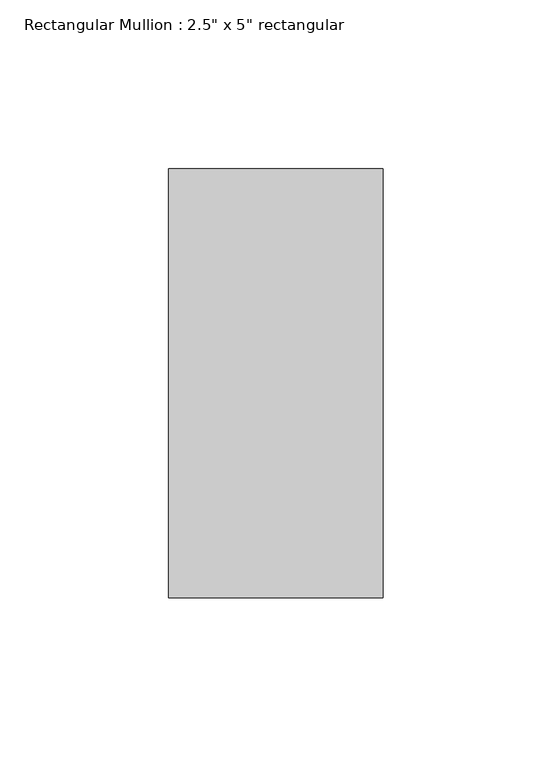
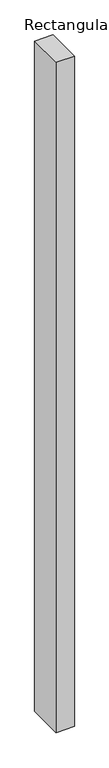
"""IFC4 building model written with IfcOpenShell, lengths in millimetres: member geometry."""

from ifc_helpers import new_model, si_unit, frame, origin, place, context, project, spatial, polyline, outline, extrude, source, transform, mapped, element, save


def member_8dcffc12(model_context):
    return source(origin(), model_context, "Body", "SweptSolid", [
        extrude(outline(polyline([(0.0, 63.5), (0.0, -63.5), (-63.5, -63.5), (-63.5, 63.5), (0.0, 63.5)])), frame((0.0, 0.0, -2445.9925421), z_axis=(0.0, 0.0, 1.0), x_axis=(1.0, 0.0, 0.0)), (0.0, 0.0, 1.0), 2445.9925421),
    ])


if __name__ == "__main__":
    model = new_model("IFC4")
    model_context = context("Model", 3, world=origin())
    ifc_project = project(units=[si_unit("LENGTHUNIT", "METRE", prefix="MILLI")], contexts=[model_context])
    site = spatial("IfcSite", under=ifc_project)
    building = spatial("IfcBuilding", under=site)
    placement = place(None, origin())
    member_shape = member_8dcffc12(model_context)
    element("IfcMember", 1, ObjectType="Rectangular Mullion : 2.5\" x 5\" rectangular", at=placement, inside=building, context=model_context, shape_type="MappedRepresentation", body=[
        mapped(member_shape, transform((0.0, 0.0, 0.0), x_axis=(1.0, 0.0, 0.0), y_axis=(0.0, 1.0, 0.0), z_axis=(0.0, 0.0, 1.0))),
    ])
    save(model, "model.ifc")

# Revit data of these elements
# Type "Rectangular Mullion : 2.5\" x 5\" rectangular"
#   built-in parameter 1007304 = 0.416667 (stored number, unit not read)
#   built-in parameter 1007301 = 0.104167 (stored number, unit not read)
#   built-in parameter 1007300 = 0.104167 (stored number, unit not read)
# Element 1 (IfcMember, "Rectangular Mullion : 2.5\" x 5\" rectangular")
#   Materials on its faces: "Aluminum"
# Materials
#   "Aluminum": class "Metal", colour RGB 247 247 247, transparency 0, Description = "Aluminum 6061", Cost = 0
